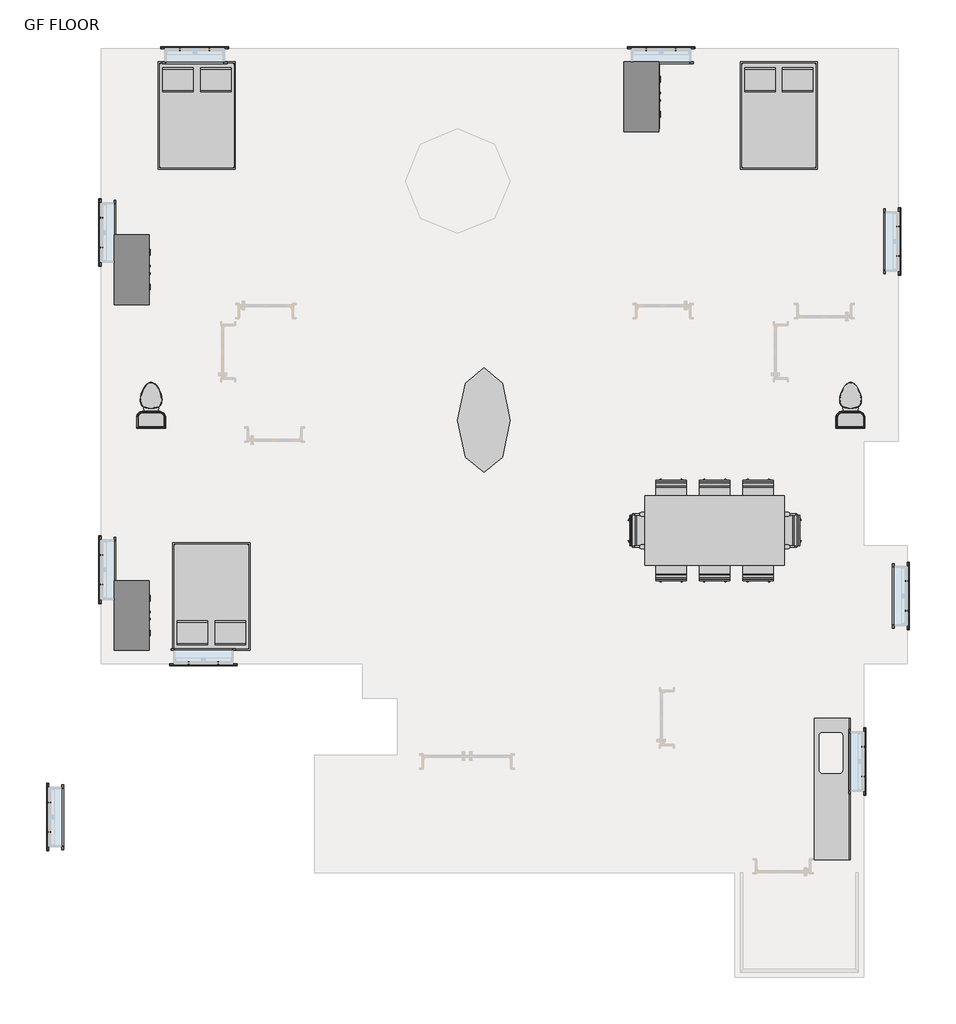
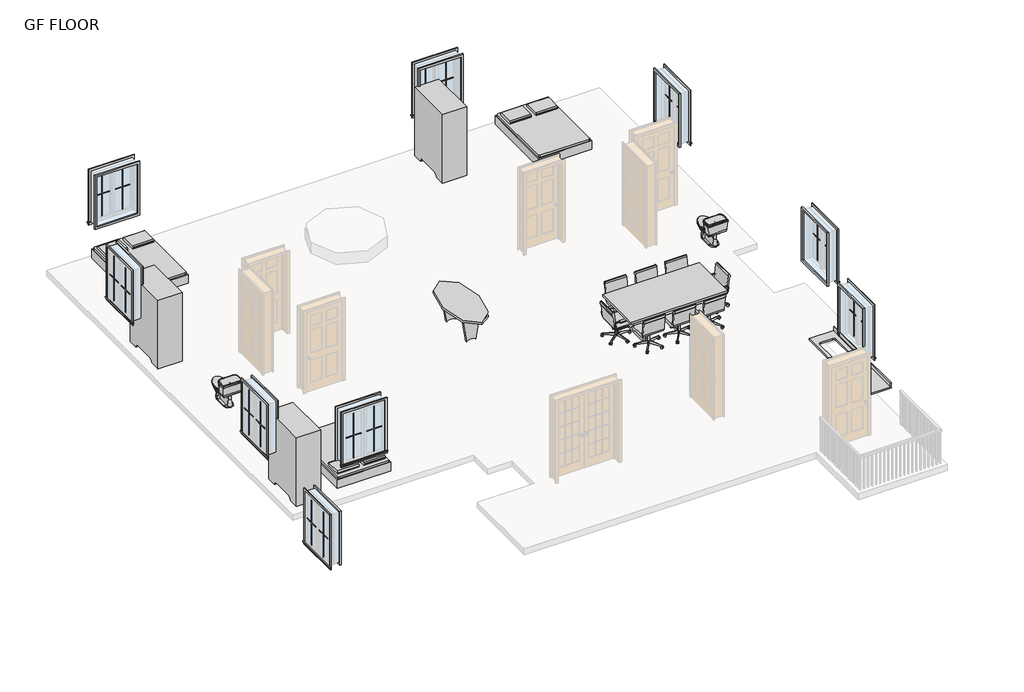
# One storey, part 2 of 2: 36 proxies, 17 furniture elements, 2 flow terminals.
"""IFC4 building model written with IfcOpenShell, lengths in millimetres."""

from ifc_helpers import new_model, si_unit, origin, place, context, project, spatial, transform, mapped, element, save
from components import muntin_pattern_2x2_muntin_pattern_2x2_88bf7f41, muntin_pattern_2x2_muntin_pattern_2x2_3dfd0a47, trim_window_exterior_flat_with_sill_4930676f, trim_window_interior_flat_picture_frame_dd064338, toilet_domestic_3d_toilet_domestic_3d_ba6479b0, toilet_domestic_3d_toilet_domestic_3d_30431060, furniture_b58f7881, chair_task_chair_task_b7f3823b, chair_task_arms_chair_task_arms_fa5a08ef, furniture_d3a4b1a9, furniture_6f689152, furniture_15aefc23, furniture_82e269c4

model = new_model("IFC4")

# Units and contexts
model_context = context("Model", 3, world=origin())
ifc_project = project(units=[si_unit("LENGTHUNIT", "METRE", prefix="MILLI")], contexts=[model_context])

# Site, building, storey
site = spatial("IfcSite", under=ifc_project)
building = spatial("IfcBuilding", under=site)
storey = spatial("IfcBuildingStorey", under=building, Name="GF FLOOR", Elevation=914.4)

# Proxies
placement = place(None, origin())
muntin_pattern_2x2_muntin_pattern_2x2_shape = muntin_pattern_2x2_muntin_pattern_2x2_88bf7f41(model_context)
element("IfcBuildingElementProxy", 1, Name="Muntin Pattern_2x2 : Muntin Pattern_2x2", ObjectType="Muntin Pattern_2x2 : Muntin Pattern_2x2", at=placement, inside=storey, context=model_context, shape_type="MappedRepresentation", body=[
    mapped(muntin_pattern_2x2_muntin_pattern_2x2_shape, transform((579.9137825, 3799.6156886, 1898.65), x_axis=(-1.0, 0.0, 0.0), y_axis=(0.0, -1.0, 0.0), z_axis=(0.0, 0.0, 1.0))),
])
element("IfcBuildingElementProxy", 2, Name="Muntin Pattern_2x2 : Muntin Pattern_2x2", ObjectType="Muntin Pattern_2x2 : Muntin Pattern_2x2", at=placement, inside=storey, context=model_context, shape_type="MappedRepresentation", body=[
    mapped(muntin_pattern_2x2_muntin_pattern_2x2_shape, transform((-1460.0237175, 5169.6281886, 1898.65), x_axis=(0.0, 1.0, 0.0), y_axis=(-1.0, 0.0, 0.0), z_axis=(0.0, 0.0, 1.0))),
])
element("IfcBuildingElementProxy", 3, Name="Muntin Pattern_2x2 : Muntin Pattern_2x2", ObjectType="Muntin Pattern_2x2 : Muntin Pattern_2x2", at=placement, inside=storey, context=model_context, shape_type="MappedRepresentation", body=[
    mapped(muntin_pattern_2x2_muntin_pattern_2x2_shape, transform((-1460.0237175, 11062.4281886, 1898.65), x_axis=(0.0, 1.0, 0.0), y_axis=(-1.0, 0.0, 0.0), z_axis=(0.0, 0.0, 1.0))),
])
element("IfcBuildingElementProxy", 4, Name="Muntin Pattern_2x2 : Muntin Pattern_2x2", ObjectType="Muntin Pattern_2x2 : Muntin Pattern_2x2", at=placement, inside=storey, context=model_context, shape_type="MappedRepresentation", body=[
    mapped(muntin_pattern_2x2_muntin_pattern_2x2_shape, transform((-90.0112175, 14524.7656886, 1898.65), x_axis=(1.0, 0.0, 0.0), y_axis=(0.0, 1.0, 0.0), z_axis=(0.0, 0.0, 1.0))),
])
element("IfcBuildingElementProxy", 5, Name="Muntin Pattern_2x2 : Muntin Pattern_2x2", ObjectType="Muntin Pattern_2x2 : Muntin Pattern_2x2", at=placement, inside=storey, context=model_context, shape_type="MappedRepresentation", body=[
    mapped(muntin_pattern_2x2_muntin_pattern_2x2_shape, transform((8063.3887825, 14524.7656886, 1898.65), x_axis=(1.0, 0.0, 0.0), y_axis=(0.0, 1.0, 0.0), z_axis=(0.0, 0.0, 1.0))),
])
element("IfcBuildingElementProxy", 6, Name="Muntin Pattern_2x2 : Muntin Pattern_2x2", ObjectType="Muntin Pattern_2x2 : Muntin Pattern_2x2", at=placement, inside=storey, context=model_context, shape_type="MappedRepresentation", body=[
    mapped(muntin_pattern_2x2_muntin_pattern_2x2_shape, transform((12465.5262825, 11427.5531886, 1898.65), x_axis=(0.0, -1.0, 0.0), y_axis=(1.0, 0.0, 0.0), z_axis=(0.0, 0.0, 1.0))),
])
element("IfcBuildingElementProxy", 7, Name="Muntin Pattern_2x2 : Muntin Pattern_2x2", ObjectType="Muntin Pattern_2x2 : Muntin Pattern_2x2", at=placement, inside=storey, context=model_context, shape_type="MappedRepresentation", body=[
    mapped(muntin_pattern_2x2_muntin_pattern_2x2_shape, transform((11855.9262825, 2334.3531886, 1898.65), x_axis=(0.0, -1.0, 0.0), y_axis=(1.0, 0.0, 0.0), z_axis=(0.0, 0.0, 1.0))),
])
element("IfcBuildingElementProxy", 8, Name="Muntin Pattern_2x2 : Muntin Pattern_2x2", ObjectType="Muntin Pattern_2x2 : Muntin Pattern_2x2", at=placement, inside=storey, context=model_context, shape_type="MappedRepresentation", body=[
    mapped(muntin_pattern_2x2_muntin_pattern_2x2_shape, transform((12617.9262825, 5229.9531886, 1898.65), x_axis=(0.0, -1.0, 0.0), y_axis=(1.0, 0.0, 0.0), z_axis=(0.0, 0.0, 1.0))),
])
element("IfcBuildingElementProxy", 9, Name="Muntin Pattern_2x2 : Muntin Pattern_2x2", ObjectType="Muntin Pattern_2x2 : Muntin Pattern_2x2", at=placement, inside=storey, context=model_context, shape_type="MappedRepresentation", body=[
    mapped(muntin_pattern_2x2_muntin_pattern_2x2_shape, transform((-2374.4237175, 845.2781886, 1898.65), x_axis=(0.0, 1.0, 0.0), y_axis=(-1.0, 0.0, 0.0), z_axis=(0.0, 0.0, 1.0))),
])
muntin_pattern_2x2_muntin_pattern_2x2_2_shape = muntin_pattern_2x2_muntin_pattern_2x2_3dfd0a47(model_context)
element("IfcBuildingElementProxy", 10, Name="Muntin Pattern_2x2 : Muntin Pattern_2x2", ObjectType="Muntin Pattern_2x2 : Muntin Pattern_2x2", at=placement, inside=storey, context=model_context, shape_type="MappedRepresentation", body=[
    mapped(muntin_pattern_2x2_muntin_pattern_2x2_2_shape, transform((62.3887825, 3799.6156886, 1898.65), x_axis=(1.0, 0.0, 0.0), y_axis=(0.0, 1.0, 0.0), z_axis=(0.0, 0.0, 1.0))),
])
element("IfcBuildingElementProxy", 11, Name="Muntin Pattern_2x2 : Muntin Pattern_2x2", ObjectType="Muntin Pattern_2x2 : Muntin Pattern_2x2", at=placement, inside=storey, context=model_context, shape_type="MappedRepresentation", body=[
    mapped(muntin_pattern_2x2_muntin_pattern_2x2_2_shape, transform((-1460.0237175, 5687.1531886, 1898.65), x_axis=(0.0, -1.0, 0.0), y_axis=(1.0, 0.0, 0.0), z_axis=(0.0, 0.0, 1.0))),
])
element("IfcBuildingElementProxy", 12, Name="Muntin Pattern_2x2 : Muntin Pattern_2x2", ObjectType="Muntin Pattern_2x2 : Muntin Pattern_2x2", at=placement, inside=storey, context=model_context, shape_type="MappedRepresentation", body=[
    mapped(muntin_pattern_2x2_muntin_pattern_2x2_2_shape, transform((-1460.0237175, 11579.9531886, 1898.65), x_axis=(0.0, -1.0, 0.0), y_axis=(1.0, 0.0, 0.0), z_axis=(0.0, 0.0, 1.0))),
])
element("IfcBuildingElementProxy", 13, Name="Muntin Pattern_2x2 : Muntin Pattern_2x2", ObjectType="Muntin Pattern_2x2 : Muntin Pattern_2x2", at=placement, inside=storey, context=model_context, shape_type="MappedRepresentation", body=[
    mapped(muntin_pattern_2x2_muntin_pattern_2x2_2_shape, transform((427.5137825, 14524.7656886, 1898.65), x_axis=(-1.0, 0.0, 0.0), y_axis=(0.0, -1.0, 0.0), z_axis=(0.0, 0.0, 1.0))),
])
element("IfcBuildingElementProxy", 14, Name="Muntin Pattern_2x2 : Muntin Pattern_2x2", ObjectType="Muntin Pattern_2x2 : Muntin Pattern_2x2", at=placement, inside=storey, context=model_context, shape_type="MappedRepresentation", body=[
    mapped(muntin_pattern_2x2_muntin_pattern_2x2_2_shape, transform((8580.9137825, 14524.7656886, 1898.65), x_axis=(-1.0, 0.0, 0.0), y_axis=(0.0, -1.0, 0.0), z_axis=(0.0, 0.0, 1.0))),
])
element("IfcBuildingElementProxy", 15, Name="Muntin Pattern_2x2 : Muntin Pattern_2x2", ObjectType="Muntin Pattern_2x2 : Muntin Pattern_2x2", at=placement, inside=storey, context=model_context, shape_type="MappedRepresentation", body=[
    mapped(muntin_pattern_2x2_muntin_pattern_2x2_2_shape, transform((12465.5262825, 10910.0281886, 1898.65), x_axis=(0.0, 1.0, 0.0), y_axis=(-1.0, 0.0, 0.0), z_axis=(0.0, 0.0, 1.0))),
])
element("IfcBuildingElementProxy", 16, Name="Muntin Pattern_2x2 : Muntin Pattern_2x2", ObjectType="Muntin Pattern_2x2 : Muntin Pattern_2x2", at=placement, inside=storey, context=model_context, shape_type="MappedRepresentation", body=[
    mapped(muntin_pattern_2x2_muntin_pattern_2x2_2_shape, transform((11855.9262825, 1816.8281886, 1898.65), x_axis=(0.0, 1.0, 0.0), y_axis=(-1.0, 0.0, 0.0), z_axis=(0.0, 0.0, 1.0))),
])
element("IfcBuildingElementProxy", 17, Name="Muntin Pattern_2x2 : Muntin Pattern_2x2", ObjectType="Muntin Pattern_2x2 : Muntin Pattern_2x2", at=placement, inside=storey, context=model_context, shape_type="MappedRepresentation", body=[
    mapped(muntin_pattern_2x2_muntin_pattern_2x2_2_shape, transform((12617.9262825, 4712.4281886, 1898.65), x_axis=(0.0, 1.0, 0.0), y_axis=(-1.0, 0.0, 0.0), z_axis=(0.0, 0.0, 1.0))),
])
element("IfcBuildingElementProxy", 18, Name="Muntin Pattern_2x2 : Muntin Pattern_2x2", ObjectType="Muntin Pattern_2x2 : Muntin Pattern_2x2", at=placement, inside=storey, context=model_context, shape_type="MappedRepresentation", body=[
    mapped(muntin_pattern_2x2_muntin_pattern_2x2_2_shape, transform((-2374.4237175, 1362.8031886, 1898.65), x_axis=(0.0, -1.0, 0.0), y_axis=(1.0, 0.0, 0.0), z_axis=(0.0, 0.0, 1.0))),
])
trim_window_exterior_flat_with_sill_shape = trim_window_exterior_flat_with_sill_4930676f(model_context)
element("IfcBuildingElementProxy", 19, Name="Trim-Window-Exterior-Flat : with Sill", ObjectType="Trim-Window-Exterior-Flat : with Sill", at=placement, inside=storey, context=model_context, shape_type="MappedRepresentation", body=[
    mapped(trim_window_exterior_flat_with_sill_shape, transform((321.1512825, 3790.0906886, 3175.0), x_axis=(1.0, 0.0, 0.0), y_axis=(0.0, 0.0, 1.0), z_axis=(0.0, -1.0, 0.0))),
])
element("IfcBuildingElementProxy", 20, Name="Trim-Window-Exterior-Flat : with Sill", ObjectType="Trim-Window-Exterior-Flat : with Sill", at=placement, inside=storey, context=model_context, shape_type="MappedRepresentation", body=[
    mapped(trim_window_exterior_flat_with_sill_shape, transform((-1469.5487175, 5428.3906886, 3175.0), x_axis=(0.0, -1.0, 0.0), y_axis=(0.0, 0.0, 1.0), z_axis=(-1.0, 0.0, 0.0))),
])
element("IfcBuildingElementProxy", 21, Name="Trim-Window-Exterior-Flat : with Sill", ObjectType="Trim-Window-Exterior-Flat : with Sill", at=placement, inside=storey, context=model_context, shape_type="MappedRepresentation", body=[
    mapped(trim_window_exterior_flat_with_sill_shape, transform((-1469.5487175, 11321.1906886, 3175.0), x_axis=(0.0, -1.0, 0.0), y_axis=(0.0, 0.0, 1.0), z_axis=(-1.0, 0.0, 0.0))),
])
element("IfcBuildingElementProxy", 22, Name="Trim-Window-Exterior-Flat : with Sill", ObjectType="Trim-Window-Exterior-Flat : with Sill", at=placement, inside=storey, context=model_context, shape_type="MappedRepresentation", body=[
    mapped(trim_window_exterior_flat_with_sill_shape, transform((168.7512825, 14534.2906886, 3175.0), x_axis=(-1.0, 0.0, 0.0), y_axis=(0.0, 0.0, 1.0), z_axis=(0.0, 1.0, 0.0))),
])
element("IfcBuildingElementProxy", 23, Name="Trim-Window-Exterior-Flat : with Sill", ObjectType="Trim-Window-Exterior-Flat : with Sill", at=placement, inside=storey, context=model_context, shape_type="MappedRepresentation", body=[
    mapped(trim_window_exterior_flat_with_sill_shape, transform((8322.1512825, 14534.2906886, 3175.0), x_axis=(-1.0, 0.0, 0.0), y_axis=(0.0, 0.0, 1.0), z_axis=(0.0, 1.0, 0.0))),
])
element("IfcBuildingElementProxy", 24, Name="Trim-Window-Exterior-Flat : with Sill", ObjectType="Trim-Window-Exterior-Flat : with Sill", at=placement, inside=storey, context=model_context, shape_type="MappedRepresentation", body=[
    mapped(trim_window_exterior_flat_with_sill_shape, transform((12475.0512825, 11168.7906886, 3175.0), x_axis=(0.0, 1.0, 0.0), y_axis=(0.0, 0.0, 1.0), z_axis=(1.0, 0.0, 0.0))),
])
element("IfcBuildingElementProxy", 25, Name="Trim-Window-Exterior-Flat : with Sill", ObjectType="Trim-Window-Exterior-Flat : with Sill", at=placement, inside=storey, context=model_context, shape_type="MappedRepresentation", body=[
    mapped(trim_window_exterior_flat_with_sill_shape, transform((11865.4512825, 2075.5906886, 3175.0), x_axis=(0.0, 1.0, 0.0), y_axis=(0.0, 0.0, 1.0), z_axis=(1.0, 0.0, 0.0))),
])
element("IfcBuildingElementProxy", 26, Name="Trim-Window-Exterior-Flat : with Sill", ObjectType="Trim-Window-Exterior-Flat : with Sill", at=placement, inside=storey, context=model_context, shape_type="MappedRepresentation", body=[
    mapped(trim_window_exterior_flat_with_sill_shape, transform((12627.4512825, 4971.1906886, 3175.0), x_axis=(0.0, 1.0, 0.0), y_axis=(0.0, 0.0, 1.0), z_axis=(1.0, 0.0, 0.0))),
])
element("IfcBuildingElementProxy", 27, Name="Trim-Window-Exterior-Flat : with Sill", ObjectType="Trim-Window-Exterior-Flat : with Sill", at=placement, inside=storey, context=model_context, shape_type="MappedRepresentation", body=[
    mapped(trim_window_exterior_flat_with_sill_shape, transform((-2383.9487175, 1104.0406886, 3175.0), x_axis=(0.0, -1.0, 0.0), y_axis=(0.0, 0.0, 1.0), z_axis=(-1.0, 0.0, 0.0))),
])
trim_window_interior_flat_picture_frame_shape = trim_window_interior_flat_picture_frame_dd064338(model_context)
element("IfcBuildingElementProxy", 28, Name="Trim-Window-Interior-Flat : Picture Frame", ObjectType="Trim-Window-Interior-Flat : Picture Frame", at=placement, inside=storey, context=model_context, shape_type="MappedRepresentation", body=[
    mapped(trim_window_interior_flat_picture_frame_shape, transform((321.1512825, 4018.6906886, 3175.0), x_axis=(-1.0, 0.0, 0.0), y_axis=(0.0, 0.0, 1.0), z_axis=(0.0, 1.0, 0.0))),
])
element("IfcBuildingElementProxy", 29, Name="Trim-Window-Interior-Flat : Picture Frame", ObjectType="Trim-Window-Interior-Flat : Picture Frame", at=placement, inside=storey, context=model_context, shape_type="MappedRepresentation", body=[
    mapped(trim_window_interior_flat_picture_frame_shape, transform((-1240.9487175, 5428.3906886, 3175.0), x_axis=(0.0, 1.0, 0.0), y_axis=(0.0, 0.0, 1.0), z_axis=(1.0, 0.0, 0.0))),
])
element("IfcBuildingElementProxy", 30, Name="Trim-Window-Interior-Flat : Picture Frame", ObjectType="Trim-Window-Interior-Flat : Picture Frame", at=placement, inside=storey, context=model_context, shape_type="MappedRepresentation", body=[
    mapped(trim_window_interior_flat_picture_frame_shape, transform((-1240.9487175, 11321.1906886, 3175.0), x_axis=(0.0, 1.0, 0.0), y_axis=(0.0, 0.0, 1.0), z_axis=(1.0, 0.0, 0.0))),
])
element("IfcBuildingElementProxy", 31, Name="Trim-Window-Interior-Flat : Picture Frame", ObjectType="Trim-Window-Interior-Flat : Picture Frame", at=placement, inside=storey, context=model_context, shape_type="MappedRepresentation", body=[
    mapped(trim_window_interior_flat_picture_frame_shape, transform((168.7512825, 14305.6906886, 3175.0), x_axis=(1.0, 0.0, 0.0), y_axis=(0.0, 0.0, 1.0), z_axis=(0.0, -1.0, 0.0))),
])
element("IfcBuildingElementProxy", 32, Name="Trim-Window-Interior-Flat : Picture Frame", ObjectType="Trim-Window-Interior-Flat : Picture Frame", at=placement, inside=storey, context=model_context, shape_type="MappedRepresentation", body=[
    mapped(trim_window_interior_flat_picture_frame_shape, transform((8322.1512825, 14305.6906886, 3175.0), x_axis=(1.0, 0.0, 0.0), y_axis=(0.0, 0.0, 1.0), z_axis=(0.0, -1.0, 0.0))),
])
element("IfcBuildingElementProxy", 33, Name="Trim-Window-Interior-Flat : Picture Frame", ObjectType="Trim-Window-Interior-Flat : Picture Frame", at=placement, inside=storey, context=model_context, shape_type="MappedRepresentation", body=[
    mapped(trim_window_interior_flat_picture_frame_shape, transform((12246.4512825, 11168.7906886, 3175.0), x_axis=(0.0, -1.0, 0.0), y_axis=(0.0, 0.0, 1.0), z_axis=(-1.0, 0.0, 0.0))),
])
element("IfcBuildingElementProxy", 34, Name="Trim-Window-Interior-Flat : Picture Frame", ObjectType="Trim-Window-Interior-Flat : Picture Frame", at=placement, inside=storey, context=model_context, shape_type="MappedRepresentation", body=[
    mapped(trim_window_interior_flat_picture_frame_shape, transform((11636.8512825, 2075.5906886, 3175.0), x_axis=(0.0, -1.0, 0.0), y_axis=(0.0, 0.0, 1.0), z_axis=(-1.0, 0.0, 0.0))),
])
element("IfcBuildingElementProxy", 35, Name="Trim-Window-Interior-Flat : Picture Frame", ObjectType="Trim-Window-Interior-Flat : Picture Frame", at=placement, inside=storey, context=model_context, shape_type="MappedRepresentation", body=[
    mapped(trim_window_interior_flat_picture_frame_shape, transform((12398.8512825, 4971.1906886, 3175.0), x_axis=(0.0, -1.0, 0.0), y_axis=(0.0, 0.0, 1.0), z_axis=(-1.0, 0.0, 0.0))),
])
element("IfcBuildingElementProxy", 36, Name="Trim-Window-Interior-Flat : Picture Frame", ObjectType="Trim-Window-Interior-Flat : Picture Frame", at=placement, inside=storey, context=model_context, shape_type="MappedRepresentation", body=[
    mapped(trim_window_interior_flat_picture_frame_shape, transform((-2155.3487175, 1104.0406886, 3175.0), x_axis=(0.0, 1.0, 0.0), y_axis=(0.0, 0.0, 1.0), z_axis=(1.0, 0.0, 0.0))),
])

# Flow terminals
toilet_domestic_3d_toilet_domestic_3d_shape = toilet_domestic_3d_toilet_domestic_3d_ba6479b0(model_context)
toilet_domestic_3d_toilet_domestic_3d_2_shape = toilet_domestic_3d_toilet_domestic_3d_30431060(model_context)
element("IfcFlowTerminal", 37, ObjectType="Toilet-Domestic-3D : Toilet-Domestic-3D", at=placement, inside=storey, context=model_context, shape_type="MappedRepresentation", body=[
    mapped(toilet_domestic_3d_toilet_domestic_3d_shape, transform((11636.8512825, 8399.586716, 914.4), x_axis=(-1.0, 0.0, 0.0), y_axis=(0.0, -1.0, 0.0), z_axis=(0.0, 0.0, 1.0))),
    mapped(toilet_domestic_3d_toilet_domestic_3d_2_shape, transform((11636.8512825, 8399.586716, 914.4), x_axis=(-1.0, 0.0, 0.0), y_axis=(0.0, -1.0, 0.0), z_axis=(0.0, 0.0, 1.0))),
])
element("IfcFlowTerminal", 38, ObjectType="Toilet-Domestic-3D : Toilet-Domestic-3D", at=placement, inside=storey, context=model_context, shape_type="MappedRepresentation", body=[
    mapped(toilet_domestic_3d_toilet_domestic_3d_shape, transform((-593.2487175, 8399.586716, 914.4), x_axis=(-1.0, 0.0, 0.0), y_axis=(0.0, -1.0, 0.0), z_axis=(0.0, 0.0, 1.0))),
    mapped(toilet_domestic_3d_toilet_domestic_3d_2_shape, transform((-593.2487175, 8399.586716, 914.4), x_axis=(-1.0, 0.0, 0.0), y_axis=(0.0, -1.0, 0.0), z_axis=(0.0, 0.0, 1.0))),
])

# Furniture
furniture_shape = furniture_b58f7881(model_context)
element("IfcFurniture", 39, ObjectType="Bed-Box : Double 53\" x 74\"", at=placement, inside=storey, context=model_context, shape_type="MappedRepresentation", body=[
    mapped(furniture_shape, transform((800.0037415, 4724.0611804, 914.4), x_axis=(-1.0, 0.0, 0.0), y_axis=(0.0, -1.0, 0.0), z_axis=(0.0, 0.0, 1.0))),
])
element("IfcFurniture", 40, ObjectType="Bed-Box : Double 53\" x 74\"", at=placement, inside=storey, context=model_context, shape_type="MappedRepresentation", body=[
    mapped(furniture_shape, transform((-132.3011765, 13600.3201968, 914.4), x_axis=(1.0, 0.0, 0.0), y_axis=(0.0, 1.0, 0.0), z_axis=(0.0, 0.0, 1.0))),
])
element("IfcFurniture", 41, ObjectType="Bed-Box : Double 53\" x 74\"", at=placement, inside=storey, context=model_context, shape_type="MappedRepresentation", body=[
    mapped(furniture_shape, transform((10043.1870381, 13600.3201968, 914.4), x_axis=(1.0, 0.0, 0.0), y_axis=(0.0, 1.0, 0.0), z_axis=(0.0, 0.0, 1.0))),
])
chair_task_chair_task_shape = chair_task_chair_task_b7f3823b(model_context)
element("IfcFurniture", 42, ObjectType="Chair-Task : Chair-Task", at=placement, inside=storey, context=model_context, shape_type="MappedRepresentation", body=[
    mapped(chair_task_chair_task_shape, transform((9402.9421022, 6742.7365903, 914.4), x_axis=(-1.0, 0.0, 0.0), y_axis=(0.0, -1.0, 0.0), z_axis=(0.0, 0.0, 1.0))),
])
element("IfcFurniture", 43, ObjectType="Chair-Task : Chair-Task", at=placement, inside=storey, context=model_context, shape_type="MappedRepresentation", body=[
    mapped(chair_task_chair_task_shape, transform((10164.9421022, 6742.7365903, 914.4), x_axis=(-1.0, 0.0, 0.0), y_axis=(0.0, -1.0, 0.0), z_axis=(0.0, 0.0, 1.0))),
])
element("IfcFurniture", 44, ObjectType="Chair-Task : Chair-Task", at=placement, inside=storey, context=model_context, shape_type="MappedRepresentation", body=[
    mapped(chair_task_chair_task_shape, transform((9120.9604629, 5485.644787, 914.4), x_axis=(1.0, 0.0, 0.0), y_axis=(0.0, 1.0, 0.0), z_axis=(0.0, 0.0, 1.0))),
])
element("IfcFurniture", 45, ObjectType="Chair-Task : Chair-Task", at=placement, inside=storey, context=model_context, shape_type="MappedRepresentation", body=[
    mapped(chair_task_chair_task_shape, transform((9882.9604629, 5485.644787, 914.4), x_axis=(1.0, 0.0, 0.0), y_axis=(0.0, 1.0, 0.0), z_axis=(0.0, 0.0, 1.0))),
])
element("IfcFurniture", 46, ObjectType="Chair-Task : Chair-Task", at=placement, inside=storey, context=model_context, shape_type="MappedRepresentation", body=[
    mapped(chair_task_chair_task_shape, transform((8640.9421022, 6742.7365903, 914.4), x_axis=(-1.0, 0.0, 0.0), y_axis=(0.0, -1.0, 0.0), z_axis=(0.0, 0.0, 1.0))),
])
element("IfcFurniture", 47, ObjectType="Chair-Task : Chair-Task", at=placement, inside=storey, context=model_context, shape_type="MappedRepresentation", body=[
    mapped(chair_task_chair_task_shape, transform((8358.9604629, 5485.644787, 914.4), x_axis=(1.0, 0.0, 0.0), y_axis=(0.0, 1.0, 0.0), z_axis=(0.0, 0.0, 1.0))),
])
chair_task_arms_chair_task_arms_shape = chair_task_arms_chair_task_arms_fa5a08ef(model_context)
element("IfcFurniture", 48, ObjectType="Chair-Task Arms : Chair-Task Arms", at=placement, inside=storey, context=model_context, shape_type="MappedRepresentation", body=[
    mapped(chair_task_arms_chair_task_arms_shape, transform((8023.8053809, 6255.1815083, 914.4), x_axis=(0.0, -1.0, 0.0), y_axis=(1.0, 0.0, 0.0), z_axis=(0.0, 0.0, 1.0))),
])
element("IfcFurniture", 49, ObjectType="Chair-Task Arms : Chair-Task Arms", at=placement, inside=storey, context=model_context, shape_type="MappedRepresentation", body=[
    mapped(chair_task_arms_chair_task_arms_shape, transform((10500.0971842, 5973.199869, 914.4), x_axis=(0.0, 1.0, 0.0), y_axis=(-1.0, 0.0, 0.0), z_axis=(0.0, 0.0, 1.0))),
])
furniture_2_shape = furniture_d3a4b1a9(model_context)
element("IfcFurniture", 50, ObjectType="Counter Top w Sink Hole : 24\" Depth", at=placement, inside=storey, context=model_context, shape_type="MappedRepresentation", body=[
    mapped(furniture_2_shape, transform((11636.8512825, 1637.1283936, 914.4), x_axis=(0.0, -1.0, 0.0), y_axis=(1.0, 0.0, 0.0), z_axis=(0.0, 0.0, 1.0))),
])
furniture_3_shape = furniture_6f689152(model_context)
element("IfcFurniture", 51, ObjectType="Table-Conference2 w Chairs : 48\" x 144\"", at=placement, inside=storey, context=model_context, shape_type="MappedRepresentation", body=[
    mapped(furniture_3_shape, transform((9261.9512825, 6114.1906886, 914.4), x_axis=(1.0, 0.0, 0.0), y_axis=(0.0, 1.0, 0.0), z_axis=(0.0, 0.0, 1.0))),
])
furniture_4_shape = furniture_15aefc23(model_context)
element("IfcFurniture", 52, ObjectType="Table-Ellipse : 72\" x 36\"", at=placement, inside=storey, context=model_context, shape_type="MappedRepresentation", body=[
    mapped(furniture_4_shape, transform((5223.3512825, 8044.5906886, 914.4), x_axis=(0.0, 1.0, 0.0), y_axis=(-1.0, 0.0, 0.0), z_axis=(0.0, 0.0, 1.0))),
])
furniture_5_shape = furniture_82e269c4(model_context)
element("IfcFurniture", 53, ObjectType="Wardrobe : 48\" x 72\" x 24\"", at=placement, inside=storey, context=model_context, shape_type="MappedRepresentation", body=[
    mapped(furniture_5_shape, transform((-1519.887527, 4897.4839485, 914.4), x_axis=(0.0, 1.0, 0.0), y_axis=(-1.0, 0.0, 0.0), z_axis=(0.0, 0.0, 1.0))),
])
element("IfcFurniture", 54, ObjectType="Wardrobe : 48\" x 72\" x 24\"", at=placement, inside=storey, context=model_context, shape_type="MappedRepresentation", body=[
    mapped(furniture_5_shape, transform((-1519.887527, 10942.6839485, 914.4), x_axis=(0.0, 1.0, 0.0), y_axis=(-1.0, 0.0, 0.0), z_axis=(0.0, 0.0, 1.0))),
])
element("IfcFurniture", 55, ObjectType="Wardrobe : 48\" x 72\" x 24\"", at=placement, inside=storey, context=model_context, shape_type="MappedRepresentation", body=[
    mapped(furniture_5_shape, transform((7395.512473, 13965.2839485, 914.4), x_axis=(0.0, 1.0, 0.0), y_axis=(-1.0, 0.0, 0.0), z_axis=(0.0, 0.0, 1.0))),
])

save(model, "model.ifc")

# Revit data of these elements
# Type "Muntin Pattern_2x2 : Muntin Pattern_2x2"
#   Width [instance default] = 4' - 0"
#   Thickness = 0' - 0 1/2"
#   Height [instance default] = 4' - 0"
#   Distance = 0' - 0 3/4"
#   Interior Material [instance default] = none
#   Exterior Material [instance default] = none
#   Default Elevation = 0
# Type "Trim-Window-Exterior-Flat : with Sill"
#   Trim Width = 0' - 2 1/4"
#   Trim Thickness_Picture Frame = 0' - 1 1/4"
#   Trim Thickness_with Sill = 0' - 0 3/4"
#   Sill Thickness = 0' - 1 1/4"
#   Opening Width [instance default] = 2' - 0"
#   Opening Height [instance default] = 3' - 0"
#   Default Elevation = 4' - 0"
#   Sill = yes
#   Picture Frame = no
#   Trim Material [instance default] = none
# Type "Trim-Window-Interior-Flat : Picture Frame"
#   Trim Thickness_Picture Frame = 0' - 1 1/4"
#   Trim Width = 0' - 2 1/4"
#   Trim Thickness_with Sill = 0' - 0 3/4"
#   Sill Thickness = 0' - 1 1/4"
#   Opening Width [instance default] = 2' - 0"
#   Opening Height [instance default] = 3' - 0"
#   Default Elevation = 4' - 0"
#   Sill = no
#   Picture Frame = yes
#   Trim Material [instance default] = none
# Type "Toilet-Domestic-3D : Toilet-Domestic-3D"
#   Assembly Code = "D2010110"
#   Toilet - Bowl/Basin Material = Porcelain, Linen
#   Toilet - Seat Material = Laminate, Linen, Matte
#   Default Elevation = 0
# Type "Bed-Box : Double 53\" x 74\""
#   Assembly Code = "E2020200"
#   Length = 6' - 2"
#   Width = 4' - 5"
#   Frame Material = Birch
#   Mattress Material = Linen, White
#   Default Elevation = 0
# Type "Chair-Task : Chair-Task"
#   Assembly Code = "E2020200"
#   Base Material = Plastic - Black
#   Caster Material = Plastic - Black
#   Seat/Back Material = Textile - Slate Blue
#   Default Elevation = 0
# Type "Chair-Task Arms : Chair-Task Arms"
#   Assembly Code = "E2020200"
#   Base Material = Plastic - Black
#   Caster Material = Plastic - Black
#   Seat/Back Material = Textile - Slate Blue
#   Default Elevation = 0
# Type "Counter Top w Sink Hole : 24\" Depth"
#   Assembly Code = "C1030400"
#   Counter Thickness = 0' - 1 1/2"
#   Depth = 2' - 1"
#   Height = 3' - 0"
#   Length [instance default] = 8' - 0"
#   Sink Location [instance default] = 2' - 0"
#   Sink Location To Wall [instance default] = 0' - 6"
#   Sink Opening Depth [instance default] = 1' - 3"
#   Sink Opening Width [instance default] = 2' - 3"
#   Counter Top Material = none
#   Default Elevation = 0
# Type "Table-Conference2 w Chairs : 48\" x 144\""
#   Assembly Code = "E2020200"
#   Description = "Seating 12-14"
#   Height = 2' - 6"
#   Length = 8' - 0"
#   Width = 4' - 0"
#   Number Of Chairs One Side = 3
#   Number Of Chairs = 8
#   Material = Wood - Cherry
#   Default Elevation = 0
# Type "Table-Ellipse : 72\" x 36\""
#   Assembly Code = "E2020200"
#   Half Width = 1' - 6"
#   Half Length = 3' - 0"
#   Height = 2' - 6"
#   Length = 6' - 0"
#   Width = 3' - 0"
#   Base Material = Birch
#   Top Material = Laminate - Black
#   Default Elevation = 0
# Type "Wardrobe : 48\" x 72\" x 24\""
#   Assembly Code = "E2020200"
#   Depth = 2' - 0"
#   Height = 6' - 0"
#   Width = 4' - 0"
#   Material = Wood - Mahogany
#   Default Elevation = 0
# Elements 1, 2, 3, 4, 5, 6, 7, 8, 9, 10, 11, 12, 13, 14, 15, 16, 17, 18 (IfcBuildingElementProxy, "Muntin Pattern_2x2 : Muntin Pattern_2x2")
#   Width = 1' - 3 1/8"
#   Height = 3' - 11 1/2"
#   Interior Material = Wood - Stained
#   Exterior Material = Clad - White
#   Phase Created = New Construction
#   Materials on its faces: "Clad - White", "Wood - Stained"
# Elements 19, 20, 21, 22, 23, 24, 25, 26, 27 (IfcBuildingElementProxy, "Trim-Window-Exterior-Flat : with Sill")
#   Opening Width = 3' - 5"
#   Opening Height = 4' - 5"
#   Trim Material = Clad - White
#   Phase Created = New Construction
#   Materials on its faces: "Clad - White"
# Elements 28, 29, 30, 31, 32, 33, 34, 35, 36 (IfcBuildingElementProxy, "Trim-Window-Interior-Flat : Picture Frame")
#   Opening Width = 3' - 5"
#   Opening Height = 4' - 5"
#   Trim Material = Wood - Stained
#   Phase Created = New Construction
#   Materials on its faces: "Wood - Stained"
# Element 37 (IfcFlowTerminal, "Toilet-Domestic-3D : Toilet-Domestic-3D")
#   Mark = "1"
#   Phase Created = New Construction
#   Materials on its faces: "Porcelain, Linen", "Laminate, Linen, Matte"
# Element 38 (IfcFlowTerminal, "Toilet-Domestic-3D : Toilet-Domestic-3D")
#   Mark = "3"
#   Phase Created = New Construction
#   Materials on its faces: "Porcelain, Linen", "Laminate, Linen, Matte"
# Elements 39, 40, 41 (IfcFurniture, "Bed-Box : Double 53\" x 74\"")
#   Phase Created = New Construction
#   Materials on its faces: "Birch", "Linen, White"
# Elements 42, 43, 44, 45, 46, 47 (IfcFurniture, "Chair-Task : Chair-Task")
#   Phase Created = New Construction
#   Materials on its faces: "Plastic - Black", "Textile - Slate Blue"
# Elements 48, 49 (IfcFurniture, "Chair-Task Arms : Chair-Task Arms")
#   Phase Created = New Construction
#   Materials on its faces: "Plastic - Black", "Textile - Slate Blue"
# Element 50 (IfcFurniture, "Counter Top w Sink Hole : 24\" Depth")
#   Sink Opening Width = 2' - 3"
#   Sink Opening Depth = 1' - 3"
#   Sink Location To Wall = 0' - 6"
#   Sink Location = 2' - 0"
#   Length = 8' - 1 1/2"
#   Phase Created = New Construction
#   Materials on its faces: "Counter Top"
# Element 51 (IfcFurniture, "Table-Conference2 w Chairs : 48\" x 144\"")
#   Phase Created = New Construction
#   Materials on its faces: "Wood - Cherry"
# Element 52 (IfcFurniture, "Table-Ellipse : 72\" x 36\"")
#   Phase Created = New Construction
#   Materials on its faces: "Birch", "Laminate - Black"
# Elements 53, 54, 55 (IfcFurniture, "Wardrobe : 48\" x 72\" x 24\"")
#   Phase Created = New Construction
#   Materials on its faces: "Wood - Mahogany"
# Materials
#   "Porcelain, Linen": class "Ceramic", colour RGB 249 239 230, transparency 0, Description = "Porcelain, linen", Cost = 0
#   "Laminate, Linen, Matte": class "Plastic", colour RGB 249 239 230, transparency 0, Description = "Plastic Laminate - Linen, Matte", Cost = 0
#   "Birch": class "Wood", colour RGB 224 178 126, transparency 0, Description = "Betula Alleghaniensis", Cost = 0
#   "Linen, White": class "Textile", colour RGB 247 247 239, transparency 0, Description = "Linen, white", Cost = 0
#   "Plastic - Black": colour RGB 0 0 0, transparency 0.7
#   "Textile - Slate Blue": colour RGB 98 102 118, transparency 0
#   "Wood - Cherry": colour RGB 151 75 0, transparency 0
#   "Laminate - Black": colour RGB 0 0 0, transparency 0
#   "Wood - Mahogany": colour RGB 138 86 45, transparency 0
#   "Clad - White": class "Wood", colour RGB 242 242 238, transparency 0, Cost = 0
#   "Wood - Stained": class "Wood", colour RGB 224 178 126, transparency 0, Cost = 0
#   "Counter Top": class "Wood", colour RGB 226 177 128, transparency 0
